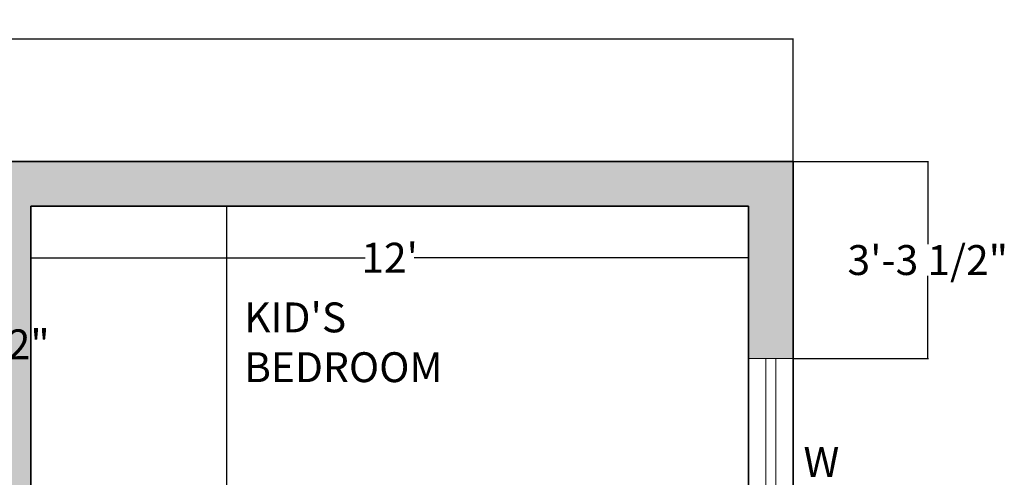
# Model space of a CAD drawing. Units: inches. Extents: x 302 to 1258, y 831 to 1373.
# Tile 13 of 13: x 1048 to 1245, y 1279 to 1371. Entities that reach past the tile are written whole.
import ezdxf

# ---------------------------------------------------------------- set-up
doc = ezdxf.new("R2010")
doc.units = ezdxf.units.IN
doc.header["$MEASUREMENT"] = 0
for name, color, linetype, lineweight in [('A-ANNO-DIMS', 2, 'Continuous', 18), ('A-ANNO-TEXT', 7, 'Continuous', 18), ('A-AREA-IDEN', 7, 'Continuous', 18), ('A-GLAZ', 4, 'Continuous', 18), ('A-WALL', 7, 'Continuous', 35), ('A-WALL-PATT', 251, 'Continuous', 13)]:
    doc.layers.add(name, color=color, linetype=linetype, lineweight=lineweight)
doc.styles.get("Standard").update_dxf_attribs({"font": 'arial.ttf'})
doc.dimstyles.get("Standard").update_dxf_attribs({"dimtxt": 6, "dimasz": 0.18, "dimexe": 0.18, "dimexo": 0.0625, "dimgap": 0.09, "dimtad": 0, "dimtih": 1, "dimtoh": 1, "dimdec": 1, "dimzin": 0, "dimdsep": 46, "dimlunit": 3, "dimtxsty": 'Standard', "dimcen": 0.09, "dimadec": 0, "dimazin": 0, "dimtfac": 1, "dimtdec": 1, "dimtofl": 0, "dimtmove": 0, "dimatfit": 3, "dimfxl": 1, "dimtolj": 1, "dimtzin": 0, "dimarcsym": 0})

# ---------------------------------------------------------------- blocks, each defined once
blk = doc.blocks.new('*D21')
at = {"layer": 'A-ANNO-DIMS', "color": 0, "lineweight": -2, "transparency": 16777216}
for p, q in [((1050.12, 1333.26), (1050.12, 1322.8)), ((1194.12, 1333.26), (1194.12, 1322.8)), ((1050.3, 1322.98), (1117.22, 1322.98)), ((1193.94, 1322.98), (1127.02, 1322.98))]:
    blk.add_line(p, q, dxfattribs=at)
at = {"layer": 'A-ANNO-DIMS', "color": 0, "transparency": 16777216}
for points in [[(1050.3, 1323.01), (1050.3, 1322.95), (1050.12, 1322.98)], [(1193.94, 1323.01), (1193.94, 1322.95), (1194.12, 1322.98)]]:
    blk.add_solid(points, dxfattribs=at)
at = {"layer": 'Defpoints', "color": 0, "transparency": 16777216}
for p in [(1050.12, 1333.32), (1194.12, 1333.32), (1194.12, 1322.98)]:
    blk.add_point(p, dxfattribs=at)
at = {"layer": 'A-ANNO-DIMS', "color": 0, "transparency": 16777216, "insert": (1122.12, 1322.98), "char_height": 6, "attachment_point": 5}
blk.add_mtext("\\A1;12'", dxfattribs=at)
blk = doc.blocks.new('*D22')
at = {"layer": 'A-ANNO-DIMS', "color": 0, "lineweight": -2, "transparency": 16777216}
for p, q in [((1194.06, 1333.32), (1089.21, 1333.32)), ((1089.39, 1333.14), (1089.39, 1276.47)), ((1089.39, 1213.5), (1089.39, 1270.17)), ((1194.06, 1213.32), (1089.21, 1213.32))]:
    blk.add_line(p, q, dxfattribs=at)
at = {"layer": 'A-ANNO-DIMS', "color": 0, "transparency": 16777216}
for points in [[(1089.36, 1333.14), (1089.42, 1333.14), (1089.39, 1333.32)], [(1089.36, 1213.5), (1089.42, 1213.5), (1089.39, 1213.32)]]:
    blk.add_solid(points, dxfattribs=at)
at = {"layer": 'Defpoints', "color": 0, "transparency": 16777216}
for p in [(1194.12, 1333.32), (1089.39, 1213.32), (1194.12, 1213.32)]:
    blk.add_point(p, dxfattribs=at)
at = {"layer": 'A-ANNO-DIMS', "color": 0, "transparency": 16777216, "insert": (1089.39, 1273.32), "char_height": 6, "attachment_point": 5}
blk.add_mtext("\\A1;10'", dxfattribs=at)
blk = doc.blocks.new('*D33')
at = {"layer": 'A-ANNO-DIMS', "color": 0, "lineweight": -2, "transparency": 16777216}
for p, q in [((846.12, 1342.38), (846.12, 1367.04)), ((846.3, 1366.86), (1010.68, 1366.86)), ((1202.94, 1366.86), (1038.56, 1366.86)), ((1203.12, 1342.38), (1203.12, 1367.04))]:
    blk.add_line(p, q, dxfattribs=at)
at = {"layer": 'A-ANNO-DIMS', "color": 0, "transparency": 16777216}
for points in [[(846.3, 1366.89), (846.3, 1366.83), (846.12, 1366.86)], [(1202.94, 1366.89), (1202.94, 1366.83), (1203.12, 1366.86)]]:
    blk.add_solid(points, dxfattribs=at)
at = {"layer": 'Defpoints', "color": 0, "transparency": 16777216}
for p in [(1203.12, 1366.86), (846.12, 1342.32), (1203.12, 1342.32)]:
    blk.add_point(p, dxfattribs=at)
at = {"layer": 'A-ANNO-DIMS', "color": 0, "transparency": 16777216, "insert": (1024.62, 1366.86), "char_height": 6, "attachment_point": 5}
blk.add_mtext('\\A1;29\'-9.0"', dxfattribs=at)
blk = doc.blocks.new('WINDOW-48IN')
for p, q in [((0, 0), (0, 9)), ((0, 9), (48, 9)), ((48, 9), (48, 0)), ((0, 5.5), (48, 5.5)), ((48, 3.5), (0, 3.5)), ((48, 0), (0, 0))]:
    blk.add_line(p, q)
blk = doc.blocks.new('*D91')
at = {"layer": 'A-ANNO-DIMS', "color": 0, "lineweight": -2, "transparency": 16777216}
for p, q in [((1203.18, 1342.32), (1230.3, 1342.32)), ((1230.12, 1342.14), (1230.12, 1325.71)), ((1230.12, 1302.89), (1230.12, 1319.32)), ((1203.18, 1302.71), (1230.3, 1302.71))]:
    blk.add_line(p, q, dxfattribs=at)
at = {"layer": 'A-ANNO-DIMS', "color": 0, "transparency": 16777216}
for points in [[(1230.09, 1342.14), (1230.15, 1342.14), (1230.12, 1342.32)], [(1230.09, 1302.89), (1230.15, 1302.89), (1230.12, 1302.71)]]:
    blk.add_solid(points, dxfattribs=at)
at = {"layer": 'Defpoints', "color": 0, "transparency": 16777216}
for p in [(1203.12, 1342.32), (1203.12, 1302.71), (1230.12, 1302.71)]:
    blk.add_point(p, dxfattribs=at)
at = {"layer": 'A-ANNO-DIMS', "color": 0, "transparency": 16777216, "insert": (1230.12, 1322.51), "char_height": 6, "attachment_point": 5}
blk.add_mtext('\\A1;3\'-3 1/2"', dxfattribs=at)
blk = doc.blocks.new('*D97')
at = {"layer": 'A-ANNO-DIMS', "color": 0, "lineweight": -2, "transparency": 16777216}
for p, q in [((974.51, 1330.32), (974.69, 1330.32)), ((974.6, 1330.23), (974.6, 1330.41)), ((1005.05, 1305.58), (993.77, 1314.74)), ((1005.23, 1305.58), (1005.05, 1305.58))]:
    blk.add_line(p, q, dxfattribs=at)
at = {"layer": 'A-ANNO-DIMS', "color": 0, "transparency": 16777216}
blk.add_solid([(993.79, 1314.77), (993.75, 1314.72), (993.63, 1314.86)], dxfattribs=at)
at = {"layer": 'Defpoints', "color": 0, "transparency": 16777216}
for p in [(974.6, 1330.32), (993.63, 1314.86)]:
    blk.add_point(p, dxfattribs=at)
at = {"layer": 'A-ANNO-DIMS', "color": 0, "transparency": 16777216, "insert": (1029.65, 1305.58), "char_height": 6, "attachment_point": 5}
blk.add_mtext('\\A1;2X R2\'-0 1/2"', dxfattribs=at)

msp = doc.modelspace()

# ---------------------------------------------------------------- hatches: boundary and pattern name
at = {"layer": 'A-WALL-PATT'}
h = msp.add_hatch(color=256, dxfattribs=at)
h.dxf.hatch_style = 1
h.paths.add_polyline_path([(1003.23, 1342.32), (934.03, 1342.32), (934.03, 1333.32), (975.12, 1333.32), (975.12, 1330.32), (979.62, 1330.32), (979.62, 1333.32), (1003.23, 1333.32)])
h.paths.add_polyline_path([(1203.12, 1342.32), (1027.23, 1342.32), (1027.23, 1333.32), (1045.62, 1333.32), (1045.62, 1213.32), (979.62, 1213.32), (979.62, 1306.32), (975.12, 1306.32), (975.12, 1213.32), (974.12, 1213.32), (974.12, 1208.82), (975.12, 1208.82), (1051.12, 1208.82), (1051.12, 1213.32), (1050.12, 1213.32), (1050.12, 1333.32), (1194.12, 1333.32), (1194.12, 1302.71), (1203.12, 1302.71)])
h.paths.add_polyline_path([(855.12, 1333.32), (886.03, 1333.32), (886.03, 1342.32), (846.12, 1342.32), (846.12, 1300.76), (855.12, 1300.76)])
h.paths.add_polyline_path([(938.12, 1213.32), (855.12, 1213.32), (855.12, 1252.76), (846.12, 1252.76), (846.12, 1164.55), (855.12, 1164.55), (855.12, 1208.82), (933.12, 1208.82), (933.12, 1082.82), (937.62, 1082.82), (937.62, 1208.82), (938.12, 1208.82)])
h.paths.add_polyline_path([(855.12, 1116.55), (846.12, 1116.55), (846.12, 1024.44), (855.12, 1024.44)])
h.paths.add_polyline_path([(855.12, 976.44), (846.12, 976.44), (846.12, 944.2), (855.12, 944.2)])

# ---------------------------------------------------------------- linework, layer by layer
at = {"layer": 'A-WALL'}
for p, q in [((846.12, 1342.32), (1203.12, 1342.32)), ((1203.12, 866.82), (1203.12, 1342.32)), ((1050.12, 1333.32), (1194.12, 1333.32)), ((1050.12, 1333.32), (1050.12, 1213.32)), ((1194.12, 1333.32), (1194.12, 1213.32))]:
    msp.add_line(p, q, dxfattribs=at)

# ---------------------------------------------------------------- block references
at = {"layer": 'A-GLAZ', "rotation": 269.9999999999991}
msp.add_blockref('WINDOW-48IN', (1194.12, 1302.71), dxfattribs=at)

# ---------------------------------------------------------------- texts
at = {"layer": 'A-ANNO-TEXT', "insert": (1205.18, 1284.96), "char_height": 6, "attachment_point": 1}
msp.add_mtext_dynamic_manual_height_columns('W', width=16.4894, gutter_width=30, heights=[0], dxfattribs=at)
at = {"layer": 'A-AREA-IDEN', "insert": (1092.92, 1313.99), "char_height": 6, "attachment_point": 1}
msp.add_mtext_dynamic_manual_height_columns("KID'S\\PBEDROOM", width=58.0496, gutter_width=30, heights=[0], dxfattribs=at)

# ---------------------------------------------------------------- dimensions: what is measured, and where the dimension line sits
at = {"layer": 'A-ANNO-DIMS'}
for base, p1, p2, picture, middle in [((1203.12, 1366.86), (846.12, 1342.32), (1203.12, 1342.32), '*D33', (1024.62, 1366.86)), ((1194.12, 1322.98), (1050.12, 1333.32), (1194.12, 1333.32), '*D21', (1122.12, 1322.98))]:
    dim = msp.add_linear_dim(base=base, p1=p1, p2=p2, dimstyle='Standard', override={"dimclrd": 0, "dimclre": 0, "dimclrt": 0}, dxfattribs=at)
    dim.commit()
    dim.dimension.update_dxf_attribs({"geometry": picture, "text_midpoint": middle})
for base, p1, p2, override, picture, middle in [((1230.12, 1302.71), (1203.12, 1342.32), (1203.12, 1302.71), {"dimdec": 1, "dimlfac": 1, "dimrnd": 0, "dimzin": 1, "dimdsep": 46, "dimlunit": 4, "dimfrac": 2}, '*D91', (1230.12, 1322.51)), ((1089.39, 1213.32), (1194.12, 1333.32), (1194.12, 1213.32), {"dimclrd": 0, "dimclre": 0, "dimclrt": 0}, '*D22', (1089.39, 1273.32))]:
    dim = msp.add_linear_dim(base=base, p1=p1, p2=p2, angle=90, dimstyle='Standard', override=override, dxfattribs=at)
    dim.commit()
    dim.dimension.update_dxf_attribs({"geometry": picture, "text_midpoint": middle})
dim = msp.add_radius_dim(center=(974.6, 1330.32), mpoint=(993.63, 1314.86), text='2X <>', dimstyle='Standard', override={"dimdec": 1, "dimlfac": 1, "dimrnd": 0, "dimzin": 1, "dimdsep": 46, "dimlunit": 4, "dimfrac": 2}, dxfattribs=at)
dim.commit()
dim.dimension.update_dxf_attribs({"geometry": '*D97', "text_midpoint": (1029.65, 1305.58), "dimtype": 164})

doc.saveas('drawing.dxf')
